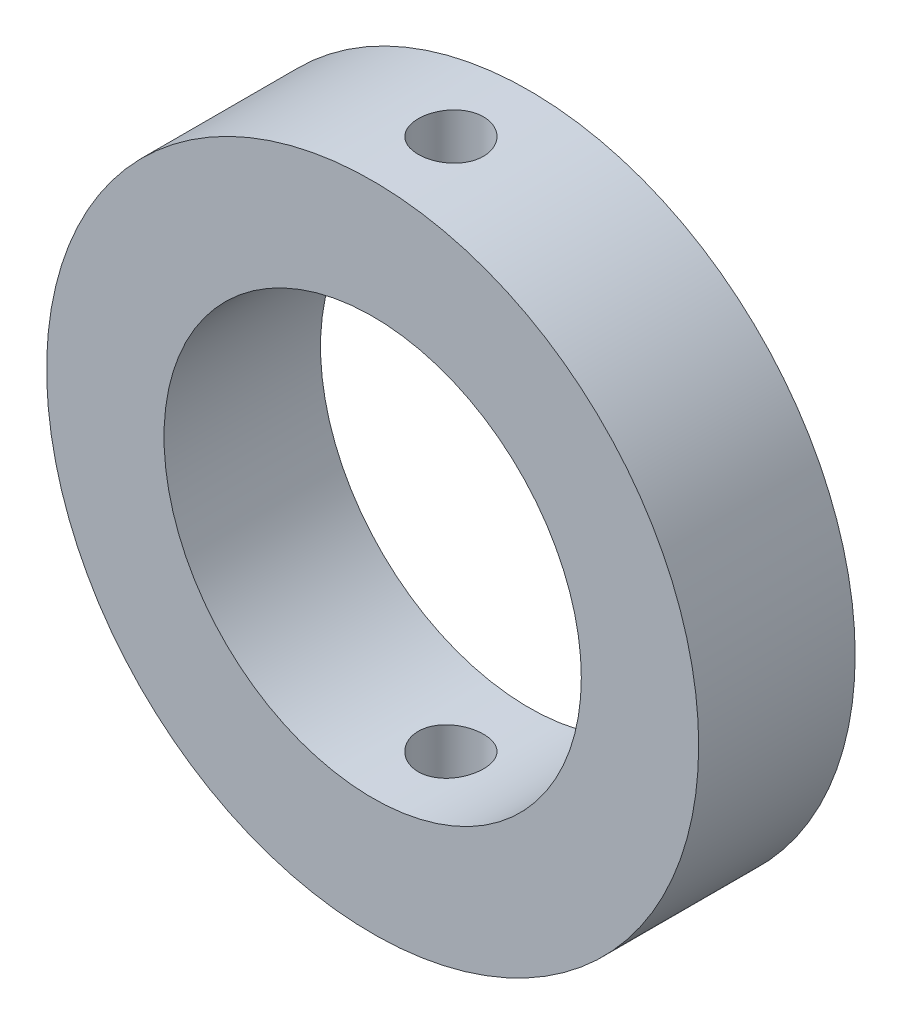
from build123d import *

# Parameters (mm, degrees)
COLLAR_RING_PROFILE_R          = 25
COLLAR_RING_PROFILE_R_2        = 16
COLLAR_RING_OD50XID32X12_DEPTH = 12
CROSS_HOLE_SKETCH_R            = 2.5
CROSS_HOLE_5_DEPTH             = 40


with BuildPart() as part:
    # Collar Ring Profile → Collar Ring OD50xID32x12 (new body)
    with BuildSketch(Plane.XY):
        Circle(COLLAR_RING_PROFILE_R)
        Circle(COLLAR_RING_PROFILE_R_2, mode=Mode.SUBTRACT)
    extrude(amount=COLLAR_RING_OD50XID32X12_DEPTH)

    # Cross Hole Sketch → Cross Hole Ø5 (cut, symmetric)
    with BuildSketch(Plane(origin=(0, 0, 0), x_dir=(1, 0, 0), z_dir=(0, 1, 0))):
        with Locations(Location((0, -6, 0), (0, 0, 270))):
            Circle(CROSS_HOLE_SKETCH_R)
    extrude(amount=CROSS_HOLE_5_DEPTH, both=True, mode=Mode.SUBTRACT)


solid = part.part
